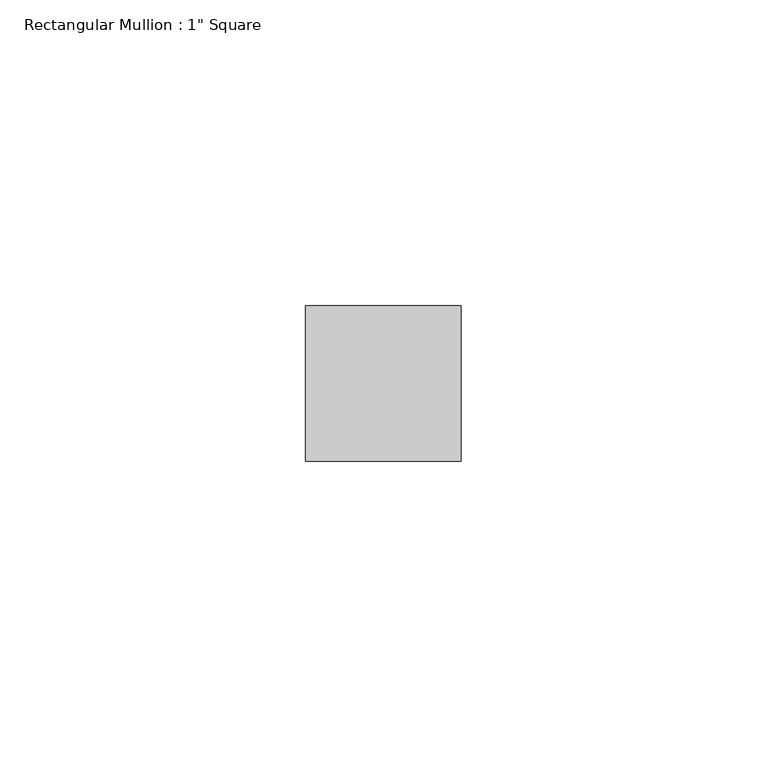
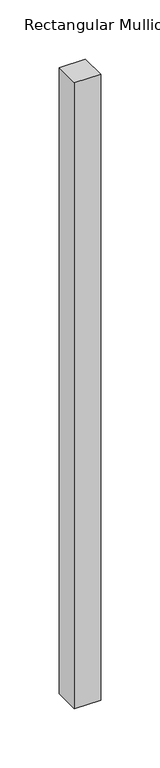
"""IFC4 building model written with IfcOpenShell, lengths in millimetres: member geometry."""

from ifc_helpers import new_model, si_unit, frame, origin, place, context, project, spatial, polyline, outline, extrude, source, transform, mapped, element, save


def member_a5642750(model_context):
    return source(origin(), model_context, "Body", "SweptSolid", [
        extrude(outline(polyline([(0.0, 12.7), (0.0, -12.7), (-25.4, -12.7), (-25.4, 12.7), (0.0, 12.7)])), frame((0.0, 0.0, -643.4666667), z_axis=(0.0, 0.0, 1.0), x_axis=(1.0, 0.0, 0.0)), (0.0, 0.0, 1.0), 643.4666667),
    ])


if __name__ == "__main__":
    model = new_model("IFC4")
    model_context = context("Model", 3, world=origin())
    ifc_project = project(units=[si_unit("LENGTHUNIT", "METRE", prefix="MILLI")], contexts=[model_context])
    site = spatial("IfcSite", under=ifc_project)
    building = spatial("IfcBuilding", under=site)
    placement = place(None, origin())
    member_shape = member_a5642750(model_context)
    element("IfcMember", 1, ObjectType="Rectangular Mullion : 1\" Square", at=placement, inside=building, context=model_context, shape_type="MappedRepresentation", body=[
        mapped(member_shape, transform((0.0, 0.0, 0.0), x_axis=(1.0, 0.0, 0.0), y_axis=(0.0, 1.0, 0.0), z_axis=(0.0, 0.0, 1.0))),
    ])
    save(model, "model.ifc")

# Revit data of these elements
# Type "Rectangular Mullion : 1\" Square"
#   built-in parameter 1007304 = 0.0833333 (stored number, unit not read)
#   built-in parameter 1007301 = 0.0416667 (stored number, unit not read)
#   built-in parameter 1007300 = 0.0416667 (stored number, unit not read)
# Element 1 (IfcMember, "Rectangular Mullion : 1\" Square")
#   Materials on its faces: "Aluminum"
# Materials
#   "Aluminum": class "Metal", colour RGB 247 247 247, transparency 0, Description = "Aluminum 6061", Cost = 0
